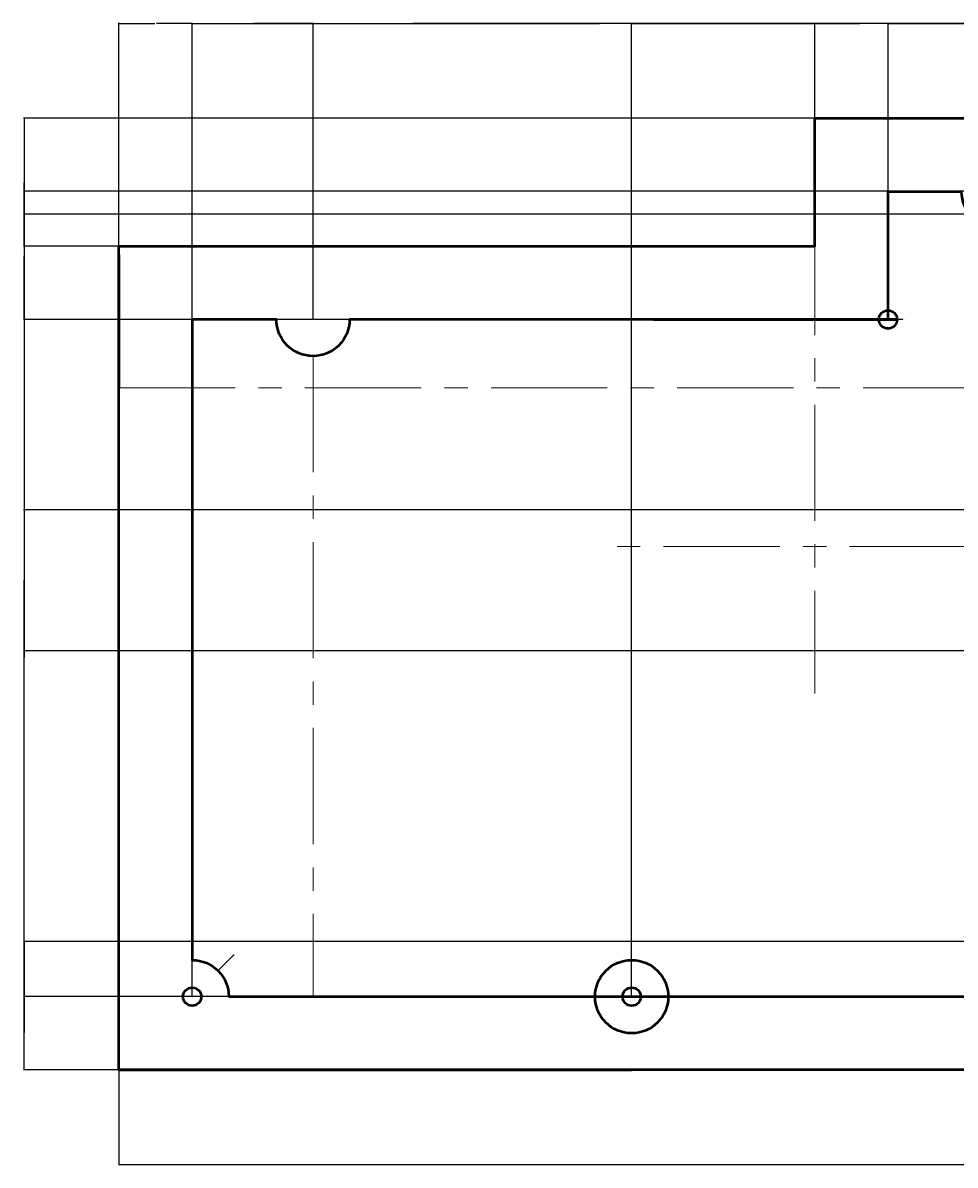
# Model space of a CAD drawing. Units: millimetres. Extents: x 2135 to 2702, y 2076 to 2388.
# Tile 1 of 2: x 2135 to 2390, y 2076 to 2388. Entities that reach past the tile are written whole.
import ezdxf

# ---------------------------------------------------------------- set-up
doc = ezdxf.new("R2010")
doc.units = ezdxf.units.MM
doc.linetypes.add('CENTER', pattern=[50.8, 31.75, -6.35, 6.35, -6.35])
for name, color, linetype, lineweight in [('M-CNTR', 4, 'CENTER', 18), ('M-DIMS', 2, 'Continuous', 18), ('M-OUTL', 7, 'Continuous', 50)]:
    doc.layers.add(name, color=color, linetype=linetype, lineweight=lineweight)
doc.styles.get("Standard").update_dxf_attribs({"font": 'arial.ttf'})
doc.dimstyles.get("Standard").update_dxf_attribs({"dimtxt": 0.18, "dimasz": 0.18, "dimexe": 0.18, "dimexo": 0.0625, "dimgap": 0.09, "dimtad": 0, "dimtih": 1, "dimtoh": 1, "dimdec": 4, "dimzin": 0, "dimdsep": 46, "dimtxsty": 'Standard', "dimcen": 0.09, "dimadec": 0, "dimazin": 0, "dimtfac": 1, "dimtdec": 4, "dimtofl": 0, "dimtmove": 0, "dimatfit": 3, "dimfxl": 1, "dimtolj": 1, "dimtzin": 0, "dimarcsym": 0})

# ---------------------------------------------------------------- blocks, each defined once
blk = doc.blocks.new('BOLT-HOLE-CBORE')
for radius in [10, 2.5]:
    blk.add_circle((10, 10), radius)
blk = doc.blocks.new('*D2')
at = {"layer": 'Defpoints', "color": 0, "transparency": 16777216}
for p in [(2676.22, 2136.75), (2161.22, 2101.69), (2676.22, 2075.84)]:
    blk.add_point(p, dxfattribs=at)
at = {"layer": 'M-DIMS', "color": 0, "lineweight": -2, "transparency": 16777216}
for p, q in [((2676.22, 2136.68), (2676.22, 2075.66)), ((2161.22, 2101.62), (2161.22, 2075.66)), ((2161.4, 2075.84), (2418.43, 2075.84)), ((2676.04, 2075.84), (2419.01, 2075.84))]:
    blk.add_line(p, q, dxfattribs=at)
at = {"layer": 'M-DIMS', "color": 0, "transparency": 16777216}
for points in [[(2161.4, 2075.87), (2161.4, 2075.81), (2161.22, 2075.84)], [(2676.04, 2075.87), (2676.04, 2075.81), (2676.22, 2075.84)]]:
    blk.add_solid(points, dxfattribs=at)
at = {"layer": 'M-DIMS', "color": 0, "transparency": 16777216, "insert": (2418.72, 2075.84), "char_height": 0.18, "attachment_point": 5}
blk.add_mtext('\\A1;515', dxfattribs=at)
blk = doc.blocks.new('*D3')
at = {"layer": 'Defpoints', "color": 0, "transparency": 16777216}
for p in [(2181.22, 2387.54), (2161.22, 2326.69), (2181.22, 2306.69)]:
    blk.add_point(p, dxfattribs=at)
at = {"layer": 'M-DIMS', "color": 0, "lineweight": -2, "transparency": 16777216}
for p, q in [((2161.22, 2326.75), (2161.22, 2387.72)), ((2161.4, 2387.54), (2171, 2387.54)), ((2181.04, 2387.54), (2171.44, 2387.54)), ((2181.22, 2306.75), (2181.22, 2387.72))]:
    blk.add_line(p, q, dxfattribs=at)
at = {"layer": 'M-DIMS', "color": 0, "transparency": 16777216}
for points in [[(2161.4, 2387.57), (2161.4, 2387.51), (2161.22, 2387.54)], [(2181.04, 2387.57), (2181.04, 2387.51), (2181.22, 2387.54)]]:
    blk.add_solid(points, dxfattribs=at)
at = {"layer": 'M-DIMS', "color": 0, "transparency": 16777216, "insert": (2171.22, 2387.54), "char_height": 0.18, "attachment_point": 5}
blk.add_mtext('\\A1;20', dxfattribs=at)
blk = doc.blocks.new('*D4')
at = {"layer": 'Defpoints', "color": 0, "transparency": 16777216}
for p in [(2351.22, 2387.54), (2351.22, 2326.69), (2181.22, 2306.69)]:
    blk.add_point(p, dxfattribs=at)
at = {"layer": 'M-DIMS', "color": 0, "lineweight": -2, "transparency": 16777216}
for p, q in [((2181.22, 2306.75), (2181.22, 2387.72)), ((2181.4, 2387.54), (2265.94, 2387.54)), ((2351.04, 2387.54), (2266.5, 2387.54)), ((2351.22, 2326.75), (2351.22, 2387.72))]:
    blk.add_line(p, q, dxfattribs=at)
at = {"layer": 'M-DIMS', "color": 0, "transparency": 16777216}
for points in [[(2181.4, 2387.57), (2181.4, 2387.51), (2181.22, 2387.54)], [(2351.04, 2387.57), (2351.04, 2387.51), (2351.22, 2387.54)]]:
    blk.add_solid(points, dxfattribs=at)
at = {"layer": 'M-DIMS', "color": 0, "transparency": 16777216, "insert": (2266.22, 2387.54), "char_height": 0.18, "attachment_point": 5}
blk.add_mtext('\\A1;170', dxfattribs=at)
blk = doc.blocks.new('*D5')
at = {"layer": 'Defpoints', "color": 0, "transparency": 16777216}
for p in [(2301.22, 2387.54), (2181.22, 2121.69), (2301.22, 2121.69)]:
    blk.add_point(p, dxfattribs=at)
at = {"layer": 'M-DIMS', "color": 0, "lineweight": -2, "transparency": 16777216}
for p, q in [((2181.22, 2121.75), (2181.22, 2387.72)), ((2181.4, 2387.54), (2240.94, 2387.54)), ((2301.04, 2387.54), (2241.5, 2387.54)), ((2301.22, 2121.75), (2301.22, 2387.72))]:
    blk.add_line(p, q, dxfattribs=at)
at = {"layer": 'M-DIMS', "color": 0, "transparency": 16777216}
for points in [[(2181.4, 2387.57), (2181.4, 2387.51), (2181.22, 2387.54)], [(2301.04, 2387.57), (2301.04, 2387.51), (2301.22, 2387.54)]]:
    blk.add_solid(points, dxfattribs=at)
at = {"layer": 'M-DIMS', "color": 0, "transparency": 16777216, "insert": (2241.22, 2387.54), "char_height": 0.18, "attachment_point": 5}
blk.add_mtext('\\A1;120', dxfattribs=at)
blk = doc.blocks.new('*D6')
at = {"layer": 'Defpoints', "color": 0, "transparency": 16777216}
for p in [(2426.22, 2387.54), (2301.22, 2121.69), (2426.22, 2121.69)]:
    blk.add_point(p, dxfattribs=at)
at = {"layer": 'M-DIMS', "color": 0, "lineweight": -2, "transparency": 16777216}
for p, q in [((2301.22, 2121.75), (2301.22, 2387.72)), ((2301.4, 2387.54), (2363.44, 2387.54)), ((2426.04, 2387.54), (2364, 2387.54)), ((2426.22, 2121.75), (2426.22, 2387.72))]:
    blk.add_line(p, q, dxfattribs=at)
at = {"layer": 'M-DIMS', "color": 0, "transparency": 16777216}
for points in [[(2301.4, 2387.57), (2301.4, 2387.51), (2301.22, 2387.54)], [(2426.04, 2387.57), (2426.04, 2387.51), (2426.22, 2387.54)]]:
    blk.add_solid(points, dxfattribs=at)
at = {"layer": 'M-DIMS', "color": 0, "transparency": 16777216, "insert": (2363.72, 2387.54), "char_height": 0.18, "attachment_point": 5}
blk.add_mtext('\\A1;125', dxfattribs=at)
blk = doc.blocks.new('*D11')
at = {"layer": 'Defpoints', "color": 0, "transparency": 16777216}
for p in [(2214.22, 2387.54), (2181.22, 2306.69), (2214.22, 2306.69)]:
    blk.add_point(p, dxfattribs=at)
at = {"layer": 'M-DIMS', "color": 0, "lineweight": -2, "transparency": 16777216}
for p, q in [((2181.22, 2306.75), (2181.22, 2387.72)), ((2181.4, 2387.54), (2197.5, 2387.54)), ((2214.04, 2387.54), (2197.94, 2387.54)), ((2214.22, 2306.75), (2214.22, 2387.72))]:
    blk.add_line(p, q, dxfattribs=at)
at = {"layer": 'M-DIMS', "color": 0, "transparency": 16777216}
for points in [[(2181.4, 2387.57), (2181.4, 2387.51), (2181.22, 2387.54)], [(2214.04, 2387.57), (2214.04, 2387.51), (2214.22, 2387.54)]]:
    blk.add_solid(points, dxfattribs=at)
at = {"layer": 'M-DIMS', "color": 0, "transparency": 16777216, "insert": (2197.72, 2387.54), "char_height": 0.18, "attachment_point": 5}
blk.add_mtext('\\A1;33', dxfattribs=at)
blk = doc.blocks.new('*D12')
at = {"layer": 'Defpoints', "color": 0, "transparency": 16777216}
for p in [(2371.22, 2387.54), (2214.22, 2306.69), (2371.22, 2306.69)]:
    blk.add_point(p, dxfattribs=at)
at = {"layer": 'M-DIMS', "color": 0, "lineweight": -2, "transparency": 16777216}
for p, q in [((2214.22, 2306.75), (2214.22, 2387.72)), ((2214.4, 2387.54), (2292.44, 2387.54)), ((2371.04, 2387.54), (2293, 2387.54)), ((2371.22, 2306.75), (2371.22, 2387.72))]:
    blk.add_line(p, q, dxfattribs=at)
at = {"layer": 'M-DIMS', "color": 0, "transparency": 16777216}
for points in [[(2214.4, 2387.57), (2214.4, 2387.51), (2214.22, 2387.54)], [(2371.04, 2387.57), (2371.04, 2387.51), (2371.22, 2387.54)]]:
    blk.add_solid(points, dxfattribs=at)
at = {"layer": 'M-DIMS', "color": 0, "transparency": 16777216, "insert": (2292.72, 2387.54), "char_height": 0.18, "attachment_point": 5}
blk.add_mtext('\\A1;157', dxfattribs=at)
blk = doc.blocks.new('*D13')
at = {"layer": 'Defpoints', "color": 0, "transparency": 16777216}
for p in [(2401.22, 2387.54), (2371.22, 2341.69), (2401.22, 2341.69)]:
    blk.add_point(p, dxfattribs=at)
at = {"layer": 'M-DIMS', "color": 0, "lineweight": -2, "transparency": 16777216}
for p, q in [((2371.22, 2341.75), (2371.22, 2387.72)), ((2371.4, 2387.54), (2386, 2387.54)), ((2401.04, 2387.54), (2386.44, 2387.54)), ((2401.22, 2341.75), (2401.22, 2387.72))]:
    blk.add_line(p, q, dxfattribs=at)
at = {"layer": 'M-DIMS', "color": 0, "transparency": 16777216}
for points in [[(2371.4, 2387.57), (2371.4, 2387.51), (2371.22, 2387.54)], [(2401.04, 2387.57), (2401.04, 2387.51), (2401.22, 2387.54)]]:
    blk.add_solid(points, dxfattribs=at)
at = {"layer": 'M-DIMS', "color": 0, "transparency": 16777216, "insert": (2386.22, 2387.54), "char_height": 0.18, "attachment_point": 5}
blk.add_mtext('\\A1;30', dxfattribs=at)
blk = doc.blocks.new('*D19')
at = {"layer": 'Defpoints', "color": 0, "transparency": 16777216}
for p in [(2430.22, 2387.54), (2371.22, 2306.69), (2430.22, 2288.03)]:
    blk.add_point(p, dxfattribs=at)
at = {"layer": 'M-DIMS', "color": 0, "lineweight": -2, "transparency": 16777216}
for p, q in [((2371.22, 2306.75), (2371.22, 2387.72)), ((2371.4, 2387.54), (2400.5, 2387.54)), ((2430.04, 2387.54), (2400.94, 2387.54)), ((2430.22, 2288.1), (2430.22, 2387.72))]:
    blk.add_line(p, q, dxfattribs=at)
at = {"layer": 'M-DIMS', "color": 0, "transparency": 16777216}
for points in [[(2371.4, 2387.57), (2371.4, 2387.51), (2371.22, 2387.54)], [(2430.04, 2387.57), (2430.04, 2387.51), (2430.22, 2387.54)]]:
    blk.add_solid(points, dxfattribs=at)
at = {"layer": 'M-DIMS', "color": 0, "transparency": 16777216, "insert": (2400.72, 2387.54), "char_height": 0.18, "attachment_point": 5}
blk.add_mtext('\\A1;59', dxfattribs=at)
blk = doc.blocks.new('*D21')
at = {"layer": 'Defpoints', "color": 0, "transparency": 16777216}
for p in [(2135.37, 2361.69), (2351.22, 2361.69), (2161.22, 2101.69)]:
    blk.add_point(p, dxfattribs=at)
at = {"layer": 'M-DIMS', "color": 0, "lineweight": -2, "transparency": 16777216}
for p, q in [((2351.15, 2361.69), (2135.19, 2361.69)), ((2135.37, 2361.51), (2135.37, 2231.87)), ((2135.37, 2101.87), (2135.37, 2231.5)), ((2161.15, 2101.69), (2135.19, 2101.69))]:
    blk.add_line(p, q, dxfattribs=at)
at = {"layer": 'M-DIMS', "color": 0, "transparency": 16777216}
for points in [[(2135.34, 2361.51), (2135.4, 2361.51), (2135.37, 2361.69)], [(2135.34, 2101.87), (2135.4, 2101.87), (2135.37, 2101.69)]]:
    blk.add_solid(points, dxfattribs=at)
at = {"layer": 'M-DIMS', "color": 0, "transparency": 16777216, "insert": (2135.37, 2231.69), "char_height": 0.18, "attachment_point": 5}
blk.add_mtext('\\A1;260', dxfattribs=at)
blk = doc.blocks.new('*D22')
at = {"layer": 'Defpoints', "color": 0, "transparency": 16777216}
for p in [(2637.37, 2121.69), (2135.37, 2101.69), (2656.22, 2101.69)]:
    blk.add_point(p, dxfattribs=at)
at = {"layer": 'M-DIMS', "color": 0, "lineweight": -2, "transparency": 16777216}
for p, q in [((2637.3, 2121.69), (2135.19, 2121.69)), ((2135.37, 2121.51), (2135.37, 2111.87)), ((2135.37, 2101.87), (2135.37, 2111.5)), ((2656.15, 2101.69), (2135.19, 2101.69))]:
    blk.add_line(p, q, dxfattribs=at)
at = {"layer": 'M-DIMS', "color": 0, "transparency": 16777216}
for points in [[(2135.34, 2121.51), (2135.4, 2121.51), (2135.37, 2121.69)], [(2135.34, 2101.87), (2135.4, 2101.87), (2135.37, 2101.69)]]:
    blk.add_solid(points, dxfattribs=at)
at = {"layer": 'M-DIMS', "color": 0, "transparency": 16777216, "insert": (2135.37, 2111.69), "char_height": 0.18, "attachment_point": 5}
blk.add_mtext('\\A1;20', dxfattribs=at)
blk = doc.blocks.new('*D23')
at = {"layer": 'Defpoints', "color": 0, "transparency": 16777216}
for p in [(2135.37, 2306.69), (2181.22, 2306.69), (2181.22, 2121.69)]:
    blk.add_point(p, dxfattribs=at)
at = {"layer": 'M-DIMS', "color": 0, "lineweight": -2, "transparency": 16777216}
for p, q in [((2181.15, 2306.69), (2135.19, 2306.69)), ((2135.37, 2306.51), (2135.37, 2214.37)), ((2135.37, 2121.87), (2135.37, 2214)), ((2181.15, 2121.69), (2135.19, 2121.69))]:
    blk.add_line(p, q, dxfattribs=at)
at = {"layer": 'M-DIMS', "color": 0, "transparency": 16777216}
for points in [[(2135.34, 2306.51), (2135.4, 2306.51), (2135.37, 2306.69)], [(2135.34, 2121.87), (2135.4, 2121.87), (2135.37, 2121.69)]]:
    blk.add_solid(points, dxfattribs=at)
at = {"layer": 'M-DIMS', "color": 0, "transparency": 16777216, "insert": (2135.37, 2214.19), "char_height": 0.18, "attachment_point": 5}
blk.add_mtext('\\A1;185', dxfattribs=at)
blk = doc.blocks.new('*D24')
at = {"layer": 'Defpoints', "color": 0, "transparency": 16777216}
for p in [(2135.37, 2326.69), (2351.22, 2326.69), (2181.22, 2306.69)]:
    blk.add_point(p, dxfattribs=at)
at = {"layer": 'M-DIMS', "color": 0, "lineweight": -2, "transparency": 16777216}
for p, q in [((2351.15, 2326.69), (2135.19, 2326.69)), ((2135.37, 2326.51), (2135.37, 2316.87)), ((2135.37, 2306.87), (2135.37, 2316.5)), ((2181.15, 2306.69), (2135.19, 2306.69))]:
    blk.add_line(p, q, dxfattribs=at)
at = {"layer": 'M-DIMS', "color": 0, "transparency": 16777216}
for points in [[(2135.34, 2326.51), (2135.4, 2326.51), (2135.37, 2326.69)], [(2135.34, 2306.87), (2135.4, 2306.87), (2135.37, 2306.69)]]:
    blk.add_solid(points, dxfattribs=at)
at = {"layer": 'M-DIMS', "color": 0, "transparency": 16777216, "insert": (2135.37, 2316.69), "char_height": 0.18, "attachment_point": 5}
blk.add_mtext('\\A1;20', dxfattribs=at)
blk = doc.blocks.new('*D25')
at = {"layer": 'Defpoints', "color": 0, "transparency": 16777216}
for p in [(2135.37, 2361.69), (2351.22, 2361.69), (2351.22, 2326.69)]:
    blk.add_point(p, dxfattribs=at)
at = {"layer": 'M-DIMS', "color": 0, "lineweight": -2, "transparency": 16777216}
for p, q in [((2351.15, 2361.69), (2135.19, 2361.69)), ((2135.37, 2361.51), (2135.37, 2344.37)), ((2135.37, 2326.87), (2135.37, 2344)), ((2351.15, 2326.69), (2135.19, 2326.69))]:
    blk.add_line(p, q, dxfattribs=at)
at = {"layer": 'M-DIMS', "color": 0, "transparency": 16777216}
for points in [[(2135.34, 2361.51), (2135.4, 2361.51), (2135.37, 2361.69)], [(2135.34, 2326.87), (2135.4, 2326.87), (2135.37, 2326.69)]]:
    blk.add_solid(points, dxfattribs=at)
at = {"layer": 'M-DIMS', "color": 0, "transparency": 16777216, "insert": (2135.37, 2344.19), "char_height": 0.18, "attachment_point": 5}
blk.add_mtext('\\A1;35', dxfattribs=at)
blk = doc.blocks.new('*D26')
at = {"layer": 'Defpoints', "color": 0, "transparency": 16777216}
for p in [(2135.37, 2341.69), (2371.22, 2341.69), (2371.22, 2306.69)]:
    blk.add_point(p, dxfattribs=at)
at = {"layer": 'M-DIMS', "color": 0, "lineweight": -2, "transparency": 16777216}
for p, q in [((2371.15, 2341.69), (2135.19, 2341.69)), ((2135.37, 2341.51), (2135.37, 2324.37)), ((2135.37, 2306.87), (2135.37, 2324)), ((2371.15, 2306.69), (2135.19, 2306.69))]:
    blk.add_line(p, q, dxfattribs=at)
at = {"layer": 'M-DIMS', "color": 0, "transparency": 16777216}
for points in [[(2135.34, 2341.51), (2135.4, 2341.51), (2135.37, 2341.69)], [(2135.34, 2306.87), (2135.4, 2306.87), (2135.37, 2306.69)]]:
    blk.add_solid(points, dxfattribs=at)
at = {"layer": 'M-DIMS', "color": 0, "transparency": 16777216, "insert": (2135.37, 2324.19), "char_height": 0.18, "attachment_point": 5}
blk.add_mtext('\\A1;35', dxfattribs=at)
blk = doc.blocks.new('*D30')
at = {"layer": 'Defpoints', "color": 0, "transparency": 16777216}
for p in [(2135.37, 2254.68), (2656.22, 2254.68), (2656.22, 2216.19)]:
    blk.add_point(p, dxfattribs=at)
at = {"layer": 'M-DIMS', "color": 0, "lineweight": -2, "transparency": 16777216}
for p, q in [((2656.15, 2254.68), (2135.19, 2254.68)), ((2135.37, 2254.5), (2135.37, 2235.62)), ((2135.37, 2216.37), (2135.37, 2235.25)), ((2656.15, 2216.19), (2135.19, 2216.19))]:
    blk.add_line(p, q, dxfattribs=at)
at = {"layer": 'M-DIMS', "color": 0, "transparency": 16777216}
for points in [[(2135.34, 2254.5), (2135.4, 2254.5), (2135.37, 2254.68)], [(2135.34, 2216.37), (2135.4, 2216.37), (2135.37, 2216.19)]]:
    blk.add_solid(points, dxfattribs=at)
at = {"layer": 'M-DIMS', "color": 0, "transparency": 16777216, "insert": (2135.37, 2235.43), "char_height": 0.18, "attachment_point": 5}
blk.add_mtext('\\A1;38.495', dxfattribs=at)
blk = doc.blocks.new('*D31')
at = {"layer": 'Defpoints', "color": 0, "transparency": 16777216}
for p in [(2135.37, 2136.75), (2676.22, 2136.75), (2656.22, 2101.69)]:
    blk.add_point(p, dxfattribs=at)
at = {"layer": 'M-DIMS', "color": 0, "lineweight": -2, "transparency": 16777216}
for p, q in [((2676.15, 2136.75), (2135.19, 2136.75)), ((2135.37, 2136.57), (2135.37, 2119.4)), ((2135.37, 2101.87), (2135.37, 2119.03)), ((2656.15, 2101.69), (2135.19, 2101.69))]:
    blk.add_line(p, q, dxfattribs=at)
at = {"layer": 'M-DIMS', "color": 0, "transparency": 16777216}
for points in [[(2135.34, 2136.57), (2135.4, 2136.57), (2135.37, 2136.75)], [(2135.34, 2101.87), (2135.4, 2101.87), (2135.37, 2101.69)]]:
    blk.add_solid(points, dxfattribs=at)
at = {"layer": 'M-DIMS', "color": 0, "transparency": 16777216, "insert": (2135.37, 2119.22), "char_height": 0.18, "attachment_point": 5}
blk.add_mtext('\\A1;35.06', dxfattribs=at)
blk = doc.blocks.new('*D34')
at = {"layer": 'Defpoints', "color": 0, "transparency": 16777216}
for p in [(2643.72, 2341.69), (2135.37, 2335.44), (2656.22, 2335.44)]:
    blk.add_point(p, dxfattribs=at)
at = {"layer": 'M-DIMS', "color": 0, "lineweight": -2, "transparency": 16777216}
for p, q in [((2643.65, 2341.69), (2135.19, 2341.69)), ((2135.37, 2341.51), (2135.37, 2338.74)), ((2135.37, 2335.62), (2135.37, 2338.38)), ((2656.15, 2335.44), (2135.19, 2335.44))]:
    blk.add_line(p, q, dxfattribs=at)
at = {"layer": 'M-DIMS', "color": 0, "transparency": 16777216}
for points in [[(2135.34, 2341.51), (2135.4, 2341.51), (2135.37, 2341.69)], [(2135.34, 2335.62), (2135.4, 2335.62), (2135.37, 2335.44)]]:
    blk.add_solid(points, dxfattribs=at)
at = {"layer": 'M-DIMS', "color": 0, "transparency": 16777216, "insert": (2135.37, 2338.56), "char_height": 0.18, "attachment_point": 5}
blk.add_mtext('\\A1;6.25', dxfattribs=at)
blk = doc.blocks.new('*D41')
at = {"layer": 'Defpoints', "color": 0, "transparency": 16777216}
for p in [(2298.72, 2121.67), (2303.72, 2121.7)]:
    blk.add_point(p, dxfattribs=at)
at = {"layer": 'M-DIMS', "color": 0, "lineweight": -2, "transparency": 16777216}
for p, q in [((2301.13, 2121.69), (2301.31, 2121.69)), ((2301.22, 2121.6), (2301.22, 2121.78)), ((2305.22, 2121.71), (2303.9, 2121.7))]:
    blk.add_line(p, q, dxfattribs=at)
at = {"layer": 'M-DIMS', "color": 0, "transparency": 16777216}
blk.add_solid([(2303.9, 2121.73), (2303.9, 2121.67), (2303.72, 2121.7)], dxfattribs=at)
at = {"layer": 'M-DIMS', "color": 0, "transparency": 16777216, "insert": (2305.65, 2121.71), "char_height": 0.18, "attachment_point": 5}
blk.add_mtext('\\A1;3X ∅5', dxfattribs=at)
blk = doc.blocks.new('*D43')
at = {"layer": 'Defpoints', "color": 0, "transparency": 16777216}
for p in [(2178.72, 2121.67), (2183.72, 2121.7)]:
    blk.add_point(p, dxfattribs=at)
at = {"layer": 'M-DIMS', "color": 0, "lineweight": -2, "transparency": 16777216}
for p, q in [((2181.13, 2121.69), (2181.31, 2121.69)), ((2181.22, 2121.6), (2181.22, 2121.78)), ((2185.22, 2121.71), (2183.9, 2121.7))]:
    blk.add_line(p, q, dxfattribs=at)
at = {"layer": 'M-DIMS', "color": 0, "transparency": 16777216}
blk.add_solid([(2183.9, 2121.73), (2183.9, 2121.67), (2183.72, 2121.7)], dxfattribs=at)
at = {"layer": 'M-DIMS', "color": 0, "transparency": 16777216, "insert": (2185.46, 2121.71), "char_height": 0.18, "attachment_point": 5}
blk.add_mtext('\\A1;∅5', dxfattribs=at)
blk = doc.blocks.new('*D44')
at = {"layer": 'Defpoints', "color": 0, "transparency": 16777216}
for p in [(2368.72, 2306.67), (2373.72, 2306.7)]:
    blk.add_point(p, dxfattribs=at)
at = {"layer": 'M-DIMS', "color": 0, "lineweight": -2, "transparency": 16777216}
for p, q in [((2371.13, 2306.69), (2371.31, 2306.69)), ((2371.22, 2306.6), (2371.22, 2306.78)), ((2375.22, 2306.71), (2373.9, 2306.7))]:
    blk.add_line(p, q, dxfattribs=at)
at = {"layer": 'M-DIMS', "color": 0, "transparency": 16777216}
blk.add_solid([(2373.9, 2306.73), (2373.9, 2306.67), (2373.72, 2306.7)], dxfattribs=at)
at = {"layer": 'M-DIMS', "color": 0, "transparency": 16777216, "insert": (2375.46, 2306.71), "char_height": 0.18, "attachment_point": 5}
blk.add_mtext('\\A1;∅5', dxfattribs=at)
blk = doc.blocks.new('*D48')
at = {"layer": 'Defpoints', "color": 0, "transparency": 16777216}
for p in [(2188.27, 2128.77), (2181.22, 2121.69)]:
    blk.add_point(p, dxfattribs=at)
at = {"layer": 'M-DIMS', "color": 0, "lineweight": -2, "transparency": 16777216}
for p, q in [((2192.51, 2133.02), (2188.4, 2128.9)), ((2192.69, 2133.02), (2192.51, 2133.02)), ((2181.13, 2121.69), (2181.31, 2121.69)), ((2181.22, 2121.6), (2181.22, 2121.78))]:
    blk.add_line(p, q, dxfattribs=at)
at = {"layer": 'M-DIMS', "color": 0, "transparency": 16777216}
blk.add_solid([(2188.38, 2128.92), (2188.42, 2128.88), (2188.27, 2128.77)], dxfattribs=at)
at = {"layer": 'M-DIMS', "color": 0, "transparency": 16777216, "insert": (2192.99, 2133.02), "char_height": 0.18, "attachment_point": 5}
blk.add_mtext('\\A1;R10', dxfattribs=at)

msp = doc.modelspace()

# ---------------------------------------------------------------- linework, layer by layer
at = {"layer": 'M-CNTR'}
for p, q in [((2351.2172, 2334.1854), (2351.2172, 2204.5212)), ((2214.2172, 2296.6854), (2214.2172, 2121.6854)), ((2161.2172, 2288.0325), (2416.86, 2288.0325)), ((2646.4762, 2244.6854), (2292.5799, 2244.6854))]:
    msp.add_line(p, q, dxfattribs=at)
at = {"layer": 'M-OUTL'}
for p, q in [((2161.2172, 2324.3525), (2161.2172, 2288.0325)), ((2161.2172, 2101.6854), (2301.2172, 2101.6854))]:
    msp.add_line(p, q, dxfattribs=at)
for points in [[(2656.2172, 2101.6854), (2161.2172, 2101.6854), (2161.2172, 2121.6854), (2161.2172, 2324.3525), (2161.2172, 2326.6854), (2181.2172, 2326.6854), (2351.2172, 2326.6854), (2351.2172, 2341.6854), (2351.2172, 2361.6854), (2371.2172, 2361.6854), (2669.9672, 2361.6854), (2676.2172, 2349.1854), (2676.2172, 2341.6854), (2676.2172, 2136.745)], [(2307.2172, 2306.6854), (2371.2172, 2306.6854), (2373.7172, 2306.6854)]]:
    msp.add_lwpolyline(points, dxfattribs=at)
for points in [[(2371.2172, 2306.6854), (2371.2172, 2341.6854), (2391.2172, 2341.6854, 1), (2411.2172, 2341.6854), (2476.2172, 2341.6854, 1), (2496.2172, 2341.6854), (2643.7172, 2341.6854), (2656.2172, 2335.4354), (2656.2172, 2254.6821)], [(2373.7172, 2306.6854), (2224.2172, 2306.6854, -1), (2204.2172, 2306.6854), (2181.2172, 2306.6854), (2181.2172, 2266.6854), (2181.2172, 2219.7301)], [(2181.2172, 2226.6854), (2181.2172, 2131.6854, -0.41421356), (2191.2172, 2121.6854), (2637.3663, 2121.6854)]]:
    msp.add_lwpolyline(points, format="xyb", dxfattribs=at)
for centre in [(2371.2172, 2306.6854), (2181.2172, 2121.6854)]:
    msp.add_circle(centre, 2.5, dxfattribs=at)

# ---------------------------------------------------------------- block references
msp.add_blockref('BOLT-HOLE-CBORE', (2291.217, 2111.685), dxfattribs=at)

# ---------------------------------------------------------------- dimensions: what is measured, and where the dimension line sits
at = {"layer": 'M-DIMS'}
for base, p1, p2, picture, middle in [((2181.2172, 2387.5354), (2161.2172, 2326.6854), (2181.2172, 2306.6854), '*D3', (2171.2172, 2387.5354)), ((2351.2172, 2387.5354), (2181.2172, 2306.6854), (2351.2172, 2326.6854), '*D4', (2266.2172, 2387.5354)), ((2301.2172, 2387.5354), (2181.2172, 2121.6854), (2301.2172, 2121.6854), '*D5', (2241.2172, 2387.5354)), ((2214.2172, 2387.5354), (2181.2172, 2306.6854), (2214.2172, 2306.6854), '*D11', (2197.7172, 2387.5354)), ((2371.2172, 2387.5354), (2214.2172, 2306.6854), (2371.2172, 2306.6854), '*D12', (2292.7172, 2387.5354)), ((2426.2172, 2387.5354), (2301.2172, 2121.6854), (2426.2172, 2121.6854), '*D6', (2363.7172, 2387.5354)), ((2401.2172, 2387.5354), (2371.2172, 2341.6854), (2401.2172, 2341.6854), '*D13', (2386.2172, 2387.5354)), ((2430.2172, 2387.5354), (2371.2172, 2306.6854), (2430.2172, 2288.0325), '*D19', (2400.7172, 2387.5354)), ((2676.2172, 2075.8354), (2161.2172, 2101.6854), (2676.2172, 2136.745), '*D2', (2418.7172, 2075.8354))]:
    dim = msp.add_linear_dim(base=base, p1=p1, p2=p2, dimstyle='Standard', override={"dimdec": 0, "dimlfac": 1, "dimrnd": 0, "dimzin": 0, "dimdsep": 46, "dimlunit": 2}, dxfattribs=at)
    dim.commit()
    dim.dimension.update_dxf_attribs({"geometry": picture, "text_midpoint": middle})
for base, p1, p2, override, picture, middle in [((2135.3672, 2361.6854), (2161.2172, 2101.6854), (2351.2172, 2361.6854), {"dimdec": 0, "dimlfac": 1, "dimrnd": 0, "dimzin": 0, "dimdsep": 46, "dimlunit": 2}, '*D21', (2135.3672, 2231.6854)), ((2135.3672, 2361.6854), (2351.2172, 2326.6854), (2351.2172, 2361.6854), {"dimdec": 0, "dimlfac": 1, "dimrnd": 0, "dimzin": 0, "dimdsep": 46, "dimlunit": 2}, '*D25', (2135.3672, 2344.1854)), ((2135.3672, 2335.4354), (2643.7172, 2341.6854), (2656.2172, 2335.4354), {"dimdec": 2, "dimlfac": 1, "dimrnd": 0, "dimzin": 0, "dimdsep": 46, "dimlunit": 2}, '*D34', (2135.3672, 2338.5604)), ((2135.3672, 2341.6854), (2371.2172, 2306.6854), (2371.2172, 2341.6854), {"dimdec": 0, "dimlfac": 1, "dimrnd": 0, "dimzin": 0, "dimdsep": 46, "dimlunit": 2}, '*D26', (2135.3672, 2324.1854)), ((2135.3672, 2326.6854), (2181.2172, 2306.6854), (2351.2172, 2326.6854), {"dimdec": 0, "dimlfac": 1, "dimrnd": 0, "dimzin": 0, "dimdsep": 46, "dimlunit": 2}, '*D24', (2135.3672, 2316.6854)), ((2135.3672, 2306.6854), (2181.2172, 2121.6854), (2181.2172, 2306.6854), {"dimdec": 0, "dimlfac": 1, "dimrnd": 0, "dimzin": 0, "dimdsep": 46, "dimlunit": 2}, '*D23', (2135.3672, 2214.1854)), ((2135.3672, 2254.68207), (2656.2172, 2216.18662), (2656.2172, 2254.68207), {"dimdec": 3, "dimlfac": 1, "dimrnd": 0, "dimzin": 0, "dimdsep": 46, "dimlunit": 2}, '*D30', (2135.3672, 2235.43434)), ((2135.3672, 2136.745), (2656.2172, 2101.6854), (2676.2172, 2136.745), {"dimdec": 2, "dimlfac": 1, "dimrnd": 0, "dimzin": 0, "dimdsep": 46, "dimlunit": 2}, '*D31', (2135.3672, 2119.2152)), ((2135.3672, 2101.6854), (2637.3663, 2121.6854), (2656.2172, 2101.6854), {"dimdec": 0, "dimlfac": 1, "dimrnd": 0, "dimzin": 0, "dimdsep": 46, "dimlunit": 2}, '*D22', (2135.3672, 2111.6854))]:
    dim = msp.add_linear_dim(base=base, p1=p1, p2=p2, angle=90, dimstyle='Standard', override=override, dxfattribs=at)
    dim.commit()
    dim.dimension.update_dxf_attribs({"geometry": picture, "text_midpoint": middle})
for p1, p2, picture, middle in [((2368.7172, 2306.6707), (2373.7172, 2306.7001), '*D44', (2375.2171, 2306.7089)), ((2178.7172, 2121.6707), (2183.7172, 2121.7001), '*D43', (2185.2171, 2121.7089))]:
    dim = msp.add_diameter_dim_2p(p1=p1, p2=p2, dimstyle='Standard', override={"dimdec": 0, "dimlfac": 1, "dimrnd": 0, "dimzin": 0, "dimdsep": 46, "dimlunit": 2}, dxfattribs=at)
    dim.commit()
    dim.dimension.update_dxf_attribs({"geometry": picture, "text_midpoint": middle, "dimtype": 163})
dim = msp.add_radius_dim(center=(2181.2172, 2121.6854), mpoint=(2188.2724, 2128.7723), dimstyle='Standard', override={"dimdec": 0, "dimlfac": 1, "dimrnd": 0, "dimzin": 0, "dimdsep": 46, "dimlunit": 2}, dxfattribs=at)
dim.commit()
dim.dimension.update_dxf_attribs({"geometry": '*D48', "text_midpoint": (2192.9903, 2133.0244), "dimtype": 164})
dim = msp.add_diameter_dim_2p(p1=(2298.7172, 2121.6707), p2=(2303.7172, 2121.7001), text='3X <>', dimstyle='Standard', override={"dimdec": 0, "dimlfac": 1, "dimrnd": 0, "dimzin": 0, "dimdsep": 46, "dimlunit": 2}, dxfattribs=at)
dim.commit()
dim.dimension.update_dxf_attribs({"geometry": '*D41', "text_midpoint": (2305.2171, 2121.7089), "dimtype": 163})

doc.saveas('drawing.dxf')
